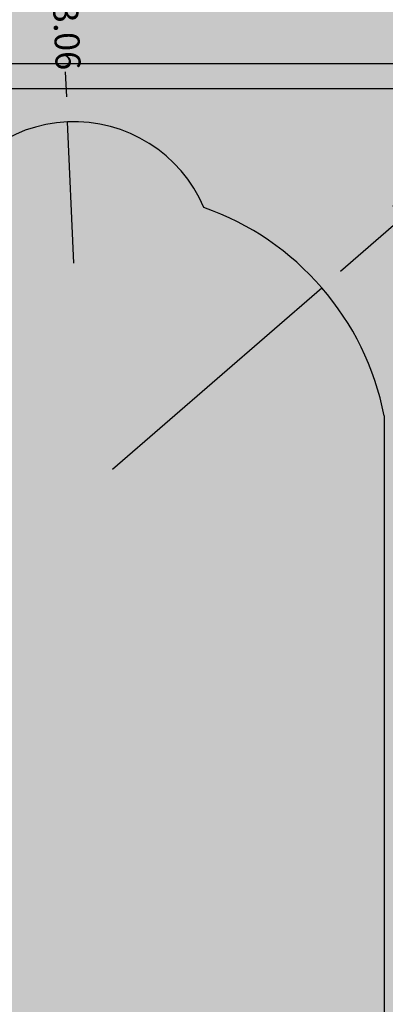
# Model space of a CAD drawing. Units: millimetres. Extents: x 78378 to 86415, y 148682 to 152721.
# Tile 8 of 18: x 80358 to 80650, y 149707 to 150495. Entities that reach past the tile are written whole.
import ezdxf

# ---------------------------------------------------------------- set-up
doc = ezdxf.new("R2010")
doc.units = ezdxf.units.MM
for name, color, linetype, lineweight in [('A-ANNO-DIMS', 2, 'Continuous', 18), ('A-FURN', 4, 'Continuous', 25), ('A-FURN-PATT', 32, 'Continuous', 13)]:
    doc.layers.add(name, color=color, linetype=linetype, lineweight=lineweight)
doc.styles.get("Standard").update_dxf_attribs({"font": 'arial.ttf'})
doc.dimstyles.new('ISO-25', dxfattribs={"dimtxt": 20, "dimasz": 20, "dimexe": 1.25, "dimexo": 0.625, "dimtad": 0, "dimdec": 1, "dimtxsty": 'Standard', "dimcen": 2.5, "dimadec": 0, "dimazin": 0, "dimtfac": 1, "dimtdec": 1, "dimtmove": 0, "dimatfit": 3, "dimfxl": 1, "dimarcsym": 0})

# ---------------------------------------------------------------- blocks, each defined once
blk = doc.blocks.new('*D32')
at = {"layer": 'A-ANNO-DIMS', "color": 0, "lineweight": -2, "transparency": 16777216}
for p, q in [((80086.404202, 150459.382643), (80086.404202, 148693.757643)), ((80692.621985, 150459.382643), (80692.621985, 148693.757643)), ((80106.404202, 148695.007643), (80355.19095843862, 148695.007643)), ((80672.621985, 148695.007643), (80423.8352285614, 148695.007643))]:
    blk.add_line(p, q, dxfattribs=at)
at = {"layer": 'A-ANNO-DIMS', "color": 0, "transparency": 16777216}
for points in [[(80106.404202, 148698.3409763333), (80106.404202, 148691.6743096666), (80086.404202, 148695.007643)], [(80672.621985, 148698.3409763333), (80672.621985, 148691.6743096666), (80692.621985, 148695.007643)]]:
    blk.add_solid(points, dxfattribs=at)
at = {"layer": 'Defpoints', "color": 0, "transparency": 16777216}
for p in [(80086.404202, 150460.007643), (80692.621985, 150460.007643), (80692.621985, 148695.007643)]:
    blk.add_point(p, dxfattribs=at)
at = {"layer": 'A-ANNO-DIMS', "color": 0, "transparency": 16777216, "insert": (80389.5130935, 148695.007643), "char_height": 20, "attachment_point": 5}
blk.add_mtext('606.2', dxfattribs=at)
blk = doc.blocks.new('*D64')
at = {"layer": 'A-ANNO-DIMS', "color": 0, "lineweight": -2, "transparency": 16777216}
for p, q in [((80660.77001983493, 150333.8066227563), (80614.48064048769, 150293.718303372)), ((80431.87671599998, 150135.576532), (80599.36214899998, 150280.625129))]:
    blk.add_line(p, q, dxfattribs=at)
at = {"layer": 'A-ANNO-DIMS', "color": 0, "transparency": 16777216}
blk.add_solid([(80612.29844475898, 150296.2380519533), (80616.66283621638, 150291.1985547907), (80599.36214899998, 150280.625129)], dxfattribs=at)
at = {"layer": 'Defpoints', "color": 0, "transparency": 16777216}
for p in [(80599.36214899998, 150280.625129), (80431.87671599998, 150135.576532)]:
    blk.add_point(p, dxfattribs=at)
at = {"layer": 'A-ANNO-DIMS', "color": 0, "transparency": 16777216, "insert": (80699.85340866249, 150367.6542870809), "char_height": 20, "attachment_point": 5, "rotation": 40.8937772563324}
blk.add_mtext('R221.56', dxfattribs=at)
blk = doc.blocks.new('*D65')
at = {"layer": 'A-ANNO-DIMS', "color": 0, "lineweight": -2, "transparency": 16777216}
for p, q in [((80394.07505015802, 150453.2874886128), (80394.982532079, 150433.3080873064)), ((80401.020132, 150300.382429), (80395.890014, 150413.328686))]:
    blk.add_line(p, q, dxfattribs=at)
at = {"layer": 'A-ANNO-DIMS', "color": 0, "transparency": 16777216}
blk.add_solid([(80398.31243229675, 150433.4593342933), (80391.65263186127, 150433.1568403196), (80395.890014, 150413.328686)], dxfattribs=at)
at = {"layer": 'Defpoints', "color": 0, "transparency": 16777216}
for p in [(80395.890014, 150413.328686), (80401.020132, 150300.382429)]:
    blk.add_point(p, dxfattribs=at)
at = {"layer": 'A-ANNO-DIMS', "color": 0, "transparency": 16777216, "insert": (80391.72908404085, 150504.937000764), "char_height": 20, "attachment_point": 5, "rotation": 272.600637092961}
blk.add_mtext('R113.06', dxfattribs=at)

msp = doc.modelspace()

# ---------------------------------------------------------------- hatches: boundary and pattern name
at = {"layer": 'A-FURN-PATT'}
h = msp.add_hatch(color=256, dxfattribs=at)
h.dxf.hatch_style = 1
h.paths.add_polyline_path([(78839.32762104142, 151040.0076434961), (78579.5199999061, 151190.0076434961), (78579.51999990609, 150470.0076434961), (78839.3276210414, 150320.0076434962)])
h.paths.add_polyline_path([(79073.15448006323, 150899.6468812434, 0.2777796948118413), (79002.26445210895, 150996.320534414, 0.7910839311940991), (78917.95668085644, 150978.871860828, 0.1804483162531181), (78856.64812911711, 150853.0137915998), (78856.6481291171, 150350.6972986685), (79073.15448006321, 150484.3179883237)])
h.paths.add_polyline_path([(79073.15448006324, 151175.0076434962), (78856.64812911711, 151050.0076434961), (78856.64812911711, 150853.0137915998, -0.1804483162531142), (78917.95668085644, 150978.871860828, -0.7910839311941295), (79002.26445210895, 150996.320534414, -0.2777796948118357), (79073.15448006323, 150899.6468812434)])
h.paths.add_polyline_path([(79341.6223552364, 151350.0076434962), (79099.13524217675, 151490.0076434961), (78596.84050798177, 151200.0076434961), (78839.32762104142, 151060.0076434961)])
h.paths.add_polyline_path([(79904.53886769625, 151675.0076434962), (79662.05175463663, 151815.0076434961), (79099.13524217677, 151490.0076434961), (79341.62235523641, 151350.0076434962)])
h.paths.add_polyline_path([(80389.51309381555, 151955.0076434962), (80389.51309381555, 152235.0076434961), (79662.05175463663, 151815.0076434961), (79904.53886769625, 151675.0076434962)])
h.paths.add_polyline_path([(80389.51309381556, 151955.0076434962), (80164.3464888316, 151825.0076434962), (80164.3464888316, 151105.0076434962), (80614.67969879952, 151105.0076434962), (80614.6796987995, 151825.0076434962)])
edge = h.paths.add_edge_path(flags=16)
edge.add_spline(control_points=[(80216.30801305865, 151728.2510436129), (80227.18536059232, 151732.9809964381), (80256.33007611947, 151745.6544105326), (80298.40995723462, 151761.9595198717), (80340.25974320961, 151805.8549546823), (80391.07708467716, 151782.0404209196), (80454.03959007034, 151805.7580622626), (80496.50068603146, 151742.4094823368), (80543.82179764508, 151733.4042954735), (80562.71817457242, 151729.808323201)], knot_values=[0, 0, 0, 0, 35.54374676083332, 95.23575346876503, 136.367675126486, 200.9329819670103, 236.7264108107793, 322.8899349763893, 380.1702736670829, 380.1702736670829, 380.1702736670829, 380.1702736670829], degree=3, periodic=0)
edge.add_line((80562.71817457242, 151729.808323201), (80562.71817457245, 151165.0076434962))
edge.add_line((80562.71817457245, 151165.0076434962), (80216.30801305866, 151165.0076434962))
edge.add_line((80216.30801305866, 151165.0076434962), (80216.30801305865, 151728.2510436129))
h.paths.add_polyline_path([(80632.00020687516, 152095.0076434962), (80389.51309381555, 152235.0076434961), (80389.51309381555, 151955.0076434962), (80614.6796987995, 151825.0076434962), (80632.0002068752, 151815.0076434962)])
h.paths.add_polyline_path([(80867.77935513339, 151958.88048878), (80632.00020687516, 152095.0076434962), (80632.0002068752, 151815.0076434962), (80632.0002068752, 151510.0076434961), (80867.77935513335, 151373.88048878)])
h.paths.add_polyline_path([(80147.02598075592, 151495.8202891389, 0.1891897896548484), (80063.56711348135, 151597.7244306894, 0.7882613551016187), (79979.26906997921, 151580.5832085911, 0.1607261321771384), (79904.53886769625, 151413.5769349066), (79904.53886769625, 150955.0076434962), (80147.0259807559, 151095.0076434962)])
h.paths.add_polyline_path([(80147.02598075592, 151815.0076434961), (79904.53886769625, 151675.0076434962), (79904.53886769625, 151413.5769349066, -0.1607261321771371), (79979.26906997921, 151580.5832085911, -0.7882613551017736), (80063.56711348135, 151597.7244306894, -0.189189789654803), (80147.02598075592, 151495.820289139)])
h.paths.add_polyline_path([(79887.21835962054, 151645.0076434962), (79640.40111954202, 151502.5076434962), (79640.40111954202, 151262.3324568555, -0.160726132177166), (79715.13132182499, 151429.33873054, -0.7882613551016538), (79799.42936532712, 151446.4799526383, -0.2129057797217132), (79887.21835962054, 151328.7246881029)])
h.paths.add_polyline_path([(79799.42936532712, 151446.4799526383, 0.7882613551016341), (79715.13132182499, 151429.33873054, 0.1607261321772164), (79640.40111954202, 151262.3324568554), (79640.401119542, 150822.5076434962), (79887.21835962054, 150965.0076434962), (79887.21835962054, 151328.7246881029, 0.2129057797217146)])
h.paths.add_polyline_path([(79605.76010339064, 151482.5076434962), (79358.94286331208, 151340.0076434962), (79358.94286331208, 151100.0700856759, -0.1607261321769527), (79433.67306559504, 151267.0763593602, -0.7882613551016573), (79517.97110909715, 151284.2175814584, -0.2129057797218584), (79605.76010339064, 151166.4623169229)])
h.paths.add_polyline_path([(79605.76010339064, 151166.4623169229, 0.2129057797218619), (79517.97110909715, 151284.2175814584, 0.7882613551016192), (79433.67306559504, 151267.0763593602, 0.160726132177026), (79358.94286331208, 151100.0700856758), (79358.9428633121, 150742.9831021798), (79419.08774136574, 150694.7323050308), (79605.76010339062, 150802.5076434962)])
edge = h.paths.add_edge_path(flags=0)
edge.add_spline(control_points=[(81152.43559504113, 151098.7675637242), (81105.72083218757, 151145.9466131586), (81038.6136018851, 151213.7208057789), (80882.38658818699, 151214.1937625951), (80797.44342369089, 151311.2996726886), (80711.86856819791, 151340.3754369685), (80681.7690729932, 151350.6023409169)], knot_values=[0, 0, 0, 0, 188.2334409997391, 270.4032751997918, 445.4517920122014, 540.4285882874335, 540.4285882874335, 540.4285882874335, 540.4285882874335], degree=3, periodic=0)
edge.add_line((80683.45384528628, 151350.0268865391), (80683.45384528628, 151104.8791667058))
edge.add_line((80683.45384528628, 151104.8791667058), (81152.43559504113, 150851.3990036113))
edge.add_line((81152.43559504113, 150851.3990036113), (81152.43559504113, 151098.7675637242))
edge = h.paths.add_edge_path(flags=0)
edge.add_spline(control_points=[(80912.90176973268, 151027.1103287246), (80892.37419951524, 151034.1027281281), (80860.16629805118, 151045.073851773), (80835.5096829066, 151068.1214310134), (80826.56785747813, 151076.4797327879)], knot_values=[0, 0, 0, 0, 63.98405104007646, 100.3914242817051, 100.3914242817051, 100.3914242817051, 100.3914242817051], degree=3, periodic=0)
edge.add_arc((80830.04136161639, 151081.2991864332), 5.940737701461331, 100.92772760250938, 234.2187380998064, ccw=False)
edge.add_spline(control_points=[(80828.91517224, 151087.1322012562), (80837.85699766847, 151078.7738994817), (80862.513612813, 151055.7263202413), (80894.72151427707, 151044.7551965964), (80915.24908449454, 151037.7627971929)], knot_values=[0, 0, 0, 0, 36.40737324162872, 100.3914242817051, 100.3914242817051, 100.3914242817051, 100.3914242817051], degree=3, periodic=0)
edge.add_arc((80914.78821288893, 151032.2794977135), 5.50263353472094, -107.95403991859422, 85.19557899478139, ccw=False)
h.paths.add_polyline_path([(81238.21798952432, 151110.0076434962), (80632.0002068752, 151460.0076434962), (80632.00020687521, 151105.0076434962), (81238.21798952432, 150755.0076434961)])
edge = h.paths.add_edge_path(flags=16)
edge.add_line((81152.43559504113, 150851.3990036113), (80683.45384528628, 151104.8791667058))
edge.add_line((80683.45384528628, 151104.8791667058), (80683.45384528628, 151350.0278851498))
edge.add_spline(control_points=[(80681.7690729932, 151350.6023409169), (80711.86856819793, 151340.3754369685), (80797.44342369087, 151311.2996726885), (80882.38658818699, 151214.1937625951), (81038.61360188508, 151213.7208057789), (81105.72083218754, 151145.9466131586), (81152.43559504113, 151098.7675637242)], knot_values=[0, 0, 0, 0, 94.97679627523202, 270.0253130876416, 352.1951472876943, 540.4285882874335, 540.4285882874335, 540.4285882874335, 540.4285882874335], degree=3, periodic=0)
edge.add_line((81152.43559504113, 151098.7675637242), (81152.43559504113, 150851.3990036113))
edge = h.paths.add_edge_path(flags=0)
edge.add_spline(control_points=[(80912.90176973268, 151027.1103287246), (80892.37419951524, 151034.1027281281), (80860.16629805118, 151045.073851773), (80835.5096829066, 151068.1214310134), (80826.56785747813, 151076.4797327879)], knot_values=[0, 0, 0, 0, 63.98405104007646, 100.3914242817051, 100.3914242817051, 100.3914242817051, 100.3914242817051], degree=3, periodic=0)
edge.add_arc((80830.04136161639, 151081.2991864332), 5.940737701461331, 100.92772760250938, 234.2187380998064, ccw=False)
edge.add_spline(control_points=[(80828.91517224, 151087.1322012562), (80837.85699766847, 151078.7738994817), (80862.513612813, 151055.7263202413), (80894.72151427707, 151044.7551965964), (80915.24908449454, 151037.7627971929)], knot_values=[0, 0, 0, 0, 36.40737324162872, 100.3914242817051, 100.3914242817051, 100.3914242817051, 100.3914242817051], degree=3, periodic=0)
edge.add_arc((80914.78821288893, 151032.2794977135), 5.50263353472094, -107.74178823087311, 85.19557899478139, ccw=False)
h.paths.add_polyline_path([(81498.02561065964, 151255.0076434964), (81238.21798952432, 151110.0076434962), (81238.21798952432, 150755.0076434961), (81498.02561065964, 150905.0076434961)])
edge = h.paths.add_edge_path(flags=16)
edge.add_spline(control_points=[(81152.43559504113, 151098.7675637242), (81105.72083218757, 151145.9466131586), (81038.6136018851, 151213.7208057789), (80882.38658818699, 151214.1937625951), (80797.44342369089, 151311.2996726886), (80711.86856819791, 151340.3754369685), (80681.7690729932, 151350.6023409169)], knot_values=[0, 0, 0, 0, 188.2334409997391, 270.4032751997918, 445.4517920122014, 540.4285882874335, 540.4285882874335, 540.4285882874335, 540.4285882874335], degree=3, periodic=0)
edge.add_line((80683.45384528628, 151350.0278851498), (80683.45384528628, 151104.8791667058))
edge.add_line((80683.45384528628, 151104.8791667058), (81152.43559504113, 150851.3990036113))
edge.add_line((81152.43559504113, 150851.3990036113), (81152.43559504113, 151098.7675637242))
h.paths.add_polyline_path([(81453.99042063669, 151280.4313723099), (80867.77935513337, 151618.8804887802), (80867.77935513335, 151373.88048878), (81238.21798952432, 151160.0076434962)])
edge = h.paths.add_edge_path(flags=16)
edge.add_line((81189.23035884998, 151297.6373231461), (81114.41656350951, 151300.215424286))
edge.add_arc((81412.09668133054, 151394.0166835757), 312.1091616570752, 179.756930250193, 197.4900342341806, ccw=False)
edge.add_ellipse((81154.0183349007, 151392.0436487034), major_axis=(-54.02641628705902, 3.630104487441717), ratio=0.22179693447735, start_angle=0, end_angle=0.351798526980474, ccw=False)
edge.add_ellipse((81154.0183349007, 151392.0436487034), major_axis=(-54.02641628705902, 3.630104487441717), ratio=0.22179693447735, start_angle=180, end_angle=359.9999999999994, ccw=False)
edge.add_spline(control_points=[(81196.1844279047, 151321.9475927373), (81224.98016894507, 151347.1455424091), (81266.88460841302, 151383.8143662904), (81222.03544587504, 151387.0303756764), (81208.00556851825, 151388.036419373)], knot_values=[0, 0, 0, 0, 75.09175173428014, 109.275804386584, 109.275804386584, 109.275804386584, 109.275804386584], degree=3, periodic=0)
edge.add_arc((80751.91118424264, 151435.614496195), 458.5692540520198, 342.489160211778, 345.646172005802, ccw=False)
edge = h.paths.add_edge_path(flags=0)
edge.add_spline(control_points=[(81196.61933933741, 151323.6570128237), (81197.89298947518, 151324.7716730423), (81199.16543060394, 151325.8857721112), (81209.0232630699, 151334.5342782859), (81217.3958880952, 151341.9835067706), (81228.09276343176, 151352.5011683344), (81231.38832729329, 151355.9523700551), (81236.9492742566, 151362.4394637984), (81239.21399888789, 151365.4773121109), (81241.49874594079, 151369.4160429918), (81242.06403714154, 151370.554153099), (81242.91869346309, 151372.6971027681), (81243.20761616631, 151373.7015371057), (81243.50116908352, 151375.5538574188), (81243.50645821408, 151376.4000030934), (81243.24316774576, 151377.9407252098), (81242.97751237078, 151378.6372898393), (81242.14015699248, 151379.9370354702), (81241.5658612394, 151380.5415506406), (81240.20389796112, 151381.5329566703), (81239.49629055885, 151381.9384109359), (81237.06189936084, 151383.0663204191), (81235.02423457924, 151383.6998500153), (81230.35196602745, 151384.7569136921), (81227.71727859117, 151385.1826462377), (81221.91180586112, 151385.9145017437), (81218.71933734383, 151386.213257908), (81213.79120700595, 151386.611489939), (81212.12519739784, 151386.7359484812), (81209.61962229511, 151386.9181059123), (81208.78653612663, 151386.9778506286), (81207.90086381555, 151387.0431786834)], knot_values=[0.0154874367935492, 0.0154874367935492, 0.0154874367935492, 0.0154874367935492, 3.337879569258078, 3.337879569258078, 25.85130624162371, 25.85130624162371, 37.52811307983364, 37.52811307983364, 49.20491991804358, 49.20491991804358, 54.285093800687, 54.285093800687, 59.36526768333043, 59.36526768333043, 64.44544156597385, 64.44544156597385, 69.52561544861727, 69.52561544861727, 74.6057893312607, 74.6057893312607, 78.49366784748545, 78.49366784748545, 86.25567095319849, 86.25567095319849, 94.01767405891154, 94.01767405891154, 102.2022655586974, 102.2022655586974, 106.2945613085904, 106.2945613085904, 108.3252217467433, 108.3252217467433, 108.3252217467433, 108.3252217467433], degree=3, periodic=0)
edge = h.paths.add_edge_path(flags=16)
edge.add_arc((81034.17317896045, 151350.4692849881), 42.58223422336468, 231.2679035139937, 306.15184603107093, ccw=False)
edge.add_line((81007.5303374241, 151317.2517344113), (81007.5303374241, 151395.1810388082))
edge.add_ellipse((81033.41196842556, 151394.7791071004), major_axis=(-25.88163100145178, 0.4537615328445103), ratio=0.2389450898152861, start_angle=0, end_angle=0.1147075293308717, ccw=False)
edge.add_ellipse((81033.41196842556, 151394.7791071004), major_axis=(-25.88163100145178, 0.4537615328445103), ratio=0.2389450898152861, start_angle=181.1677708707583, end_angle=358.9476457193874, ccw=False)
edge.add_ellipse((81033.41196842556, 151395.7791071004), major_axis=(-25.88163100145178, 0.4537615328445103), ratio=0.2389450898152861, start_angle=179.9999999981626, end_angle=360.1147075293309, ccw=False)
edge.add_ellipse((81033.41196842556, 151395.7791071004), major_axis=(-25.88163100145178, 0.4537615328445103), ratio=0.2389450898152861, start_angle=178.9476457196991, end_angle=179.9999999981626, ccw=False)
edge.add_line((81059.293599427, 151395.1778229301), (81059.293599427, 151394.3771753934))
edge.add_ellipse((81033.41196842556, 151394.7791071004), major_axis=(-25.88163100145178, 0.4537615328445103), ratio=0.2389450898152861, start_angle=179.9999999981626, end_angle=180.1147075311684, ccw=False)
edge.add_ellipse((81033.41196842556, 151394.7791071004), major_axis=(-25.88163100145178, 0.4537615328445103), ratio=0.2389450898152861, start_angle=3.6903097823663984, end_angle=176.440650305715, ccw=False)
edge.add_line((81059.293599427, 151393.3387785743), (81059.293599427, 151316.0859874871))
h.paths.add_polyline_path([(80951.93545857484, 151343.9567836094), (80909.6837602833, 151362.463470517), (80904.02186617583, 151443.961481619, -0.3813330760227573), (80987.21689667807, 151411.3716886216)], flags=16)
h = msp.add_hatch(color=256, dxfattribs=at)
h.dxf.hatch_style = 1
h.paths.add_polyline_path([(80389.81355980314, 150935.1811176149), (80389.51309381555, 151105.0076434962), (80164.3464888316, 151105.0076434962), (79904.53886769625, 150955.0076434962), (79433.58476952511, 150683.1021681411), (79459.41281351625, 150662.3818050495), (79243.9048024148, 150537.9581968276), (79160.4069246431, 150518.167363956), (78839.3276210414, 150320.0076434962), (78579.51999990609, 150470.0076434961), (78570.85974586825, 150475.0076434961), (78570.85974586825, 150465.0076434962), (78570.85974586825, 149885.0076434961)])
h.paths.add_polyline_path([(80086.40420249099, 150460.0076434961), (79826.59658135568, 150610.0076434961), (78570.85974586825, 149885.0076434961), (78830.66736700358, 149735.0076434961)])
h.paths.add_polyline_path([(79540.80006404899, 150161.0556565937), (79217.39666007676, 149974.3386142535), (78980.9165707482, 150110.8704574853), (79304.31997472048, 150297.5874998256)], flags=16)
h.paths.add_polyline_path([(79506.15904789761, 150161.0556565937), (79217.39666007677, 149994.3386142535), (79015.55758689957, 150110.8704574853), (79304.31997472048, 150277.5874998256)], flags=0)
edge = h.paths.add_edge_path(flags=0)
edge.add_arc((79247.8635885932, 150177.154059363), 137.979927152229, 256.0025927560106, 293.5594108656914)
edge.add_arc((79240.76712928673, 150078.260535577), 68.08549769177299, 336.0991039681863, 387.369687653981)
edge.add_ellipse((79258.3073696606, 150109.4851683714), major_axis=(-42.62344506003415, -1.659142297571932), ratio=0.1604284291443649, start_angle=0, end_angle=179.0977278657225, ccw=False)
edge.add_arc((79285.21118690472, 150074.2509041072), 77.20964330046426, 155.1233103751286, 203.6557939001038)
edge = h.paths.add_edge_path(flags=0)
edge.add_ellipse((79258.69578401413, 150110.8297486024), major_axis=(-42.62344506003415, -1.659142297571932), ratio=0.1604284291443649, start_angle=350.6039411592706, end_angle=356.2289762200799)
edge.add_line((79219.16897707367, 150111.8937051806), (79218.32684768032, 150109.4140931549))
edge.add_arc((79262.46751974897, 150032.9602064517), 88.28134413732826, 112.39312291994881, 119.99999999999571, ccw=False)
h.paths.add_polyline_path([(79287.06250338514, 150086.9702731333, -0.247702064009433), (79288.19674658246, 150077.2955427019, -0.3904765126137986), (79265.47309673205, 150072.5437639662, -0.4872615262363024), (79264.07897218876, 150082.3768585209, 0.3956043262328261)], flags=0)
h.paths.add_polyline_path([(80389.51309381556, 150935.0076434961), (79826.59658135568, 150610.0076434961), (80086.40420249099, 150460.0076434961), (80692.6219851401, 150460.0076434961), (80952.42960627541, 150610.0076434961)])
edge = h.paths.add_edge_path(flags=16)
edge.add_ellipse((80392.44658491029, 150825.6009587087), major_axis=(-133.0756756189512, 7.721978101297283), ratio=0.424499569836956, start_angle=0, end_angle=360)
edge = h.paths.add_edge_path(flags=0)
edge.add_spline(control_points=[(80269.35411604258, 150832.7436415815), (80269.29193278665, 150831.6720147667), (80269.35031475963, 150830.592249842), (80269.73411879689, 150828.3360718096), (80270.06118209881, 150827.1586823489), (80271.04613754865, 150824.6748448987), (80271.70517726007, 150823.3691586005), (80273.40612032128, 150820.6503360826), (80274.44810410585, 150819.2381263036), (80276.93657810257, 150816.3508564802), (80278.3827638828, 150814.8762414973), (80282.58575216534, 150811.0913237019), (80285.62609899955, 150808.7701423959), (80292.60313446997, 150804.2267034199), (80296.53882829295, 150802.0041234762), (80305.19495220963, 150797.7581273222), (80309.91505114386, 150795.7343743789), (80320.0111596611, 150791.9599857595), (80325.38703862559, 150790.2091628441), (80339.21624322617, 150786.3149836253), (80347.95776464436, 150784.3563224224), (80366.06785395242, 150781.2568288573), (80375.43585590576, 150780.1158444778), (80394.309330179, 150778.7158311894), (80403.81420373028, 150778.4568170495), (80422.465596717, 150778.8319300563), (80431.61154730739, 150779.4662025667), (80449.06079653747, 150781.5837654722), (80457.36359407243, 150783.0675039467), (80472.6698529301, 150786.7766095128), (80479.67258750588, 150789.0032721294), (80490.18936031369, 150793.2813222805), (80494.12675567923, 150795.1967122277), (80501.0145611878, 150799.188512515), (80503.9631522054, 150801.2651387212), (80508.20659370373, 150804.9015163823), (80509.7300059309, 150806.4609393726), (80512.19955536906, 150809.4942049083), (80513.14558327098, 150810.9657349426), (80514.42909982229, 150813.5430698013), (80514.84355071915, 150814.6688389962), (80515.39838138374, 150816.8624682529), (80515.5404646545, 150817.9315158847), (80515.58008082317, 150820.0980035506), (80515.47732053277, 150821.197772811), (80514.99049560675, 150823.5061778107), (80514.6046629432, 150824.7154201442), (80513.48543938114, 150827.2641302181), (80512.7510921682, 150828.6026612985), (80510.88722780815, 150831.3808578872), (80509.75776214547, 150832.8196480674), (80507.0873051963, 150835.7513330261), (80505.5466409065, 150837.243857375), (80501.06238832264, 150841.0944478958), (80497.8199298022, 150843.4575549534), (80490.4173793454, 150848.0619874995), (80486.25822277585, 150850.3037143823), (80477.14480578042, 150854.5642972019), (80472.19085006021, 150856.583496544), (80461.6274878137, 150860.3244857693), (80456.01820904585, 150862.0464562905), (80441.73317330678, 150865.8126742317), (80432.78853232553, 150867.6675482482), (80414.33909310326, 150870.5316780972), (80404.8348928345, 150871.5410542788), (80385.7706775062, 150872.6572210053), (80376.21128671143, 150872.7639759942), (80357.54439280283, 150872.0728395342), (80348.43747055416, 150871.27476178), (80331.16822413795, 150868.8299635098), (80323.00642023917, 150867.1826714935), (80309.47200145545, 150863.5363064667), (80303.8627990537, 150861.6592748057), (80293.8018064812, 150857.5400855607), (80289.35122989668, 150855.2968623192), (80282.77569843757, 150851.2345481044), (80280.34726566746, 150849.4578867352), (80276.26060564672, 150845.9127204516), (80274.60404284154, 150844.1457946164), (80272.31573199967, 150841.1242619346), (80271.53575166185, 150839.8453762844), (80270.34961441216, 150837.3878672019), (80269.94168426798, 150836.2101260174), (80269.5065140611, 150834.2814629481), (80269.3988329965, 150833.5142652193), (80269.35411604258, 150832.7436415815)], knot_values=[0, 0, 0, 0, 0.0975004598125087, 0.0975004598125087, 0.1950009196250173, 0.1950009196250173, 0.2925013794375259, 0.2925013794375259, 0.3900018392500346, 0.3900018392500346, 0.4875022990625432, 0.4875022990625432, 0.6388032241337034, 0.6388032241337034, 0.7901041492048636, 0.7901041492048636, 0.9414050742760238, 0.9414050742760238, 1.092705999347184, 1.092705999347184, 1.312817101002443, 1.312817101002443, 1.532928202657702, 1.532928202657702, 1.753039304312961, 1.753039304312961, 1.973150405968221, 1.973150405968221, 2.19326150762348, 2.19326150762348, 2.413372609278739, 2.413372609278739, 2.569860632934037, 2.569860632934037, 2.726348656589336, 2.726348656589336, 2.844186581547077, 2.844186581547077, 2.962024506504818, 2.962024506504818, 3.060233875946405, 3.060233875946405, 3.158443245387991, 3.158443245387991, 3.256652614829578, 3.256652614829578, 3.354861984271164, 3.354861984271164, 3.453071353712751, 3.453071353712751, 3.551280723154337, 3.551280723154337, 3.649490092595923, 3.649490092595923, 3.803927730406353, 3.803927730406353, 3.958365368216782, 3.958365368216782, 4.112803006027212, 4.112803006027212, 4.267240643837642, 4.267240643837642, 4.489203494974081, 4.489203494974081, 4.711166346110521, 4.711166346110521, 4.93312919724696, 4.93312919724696, 5.155092048383399, 5.155092048383399, 5.377054899519838, 5.377054899519838, 5.557853608626545, 5.557853608626545, 5.738652317733252, 5.738652317733252, 5.872395555677483, 5.872395555677483, 6.006138793621714, 6.006138793621714, 6.109604996023907, 6.109604996023907, 6.2130711984261, 6.2130711984261, 6.283185307179586, 6.283185307179586, 6.283185307179586, 6.283185307179586], degree=3, periodic=0)
edge = h.paths.add_edge_path(flags=0)
edge.add_ellipse((80392.446576265, 150825.6009639553), major_axis=(-101.8397670786795, 3.392257208815831), ratio=0.403492477068114, start_angle=0, end_angle=360)
edge = h.paths.add_edge_path(flags=0)
edge.add_ellipse((80391.1657165424, 150858.3745518381), major_axis=(9.088237780547283, -0.67334552975693), ratio=0.3513541290445306, start_angle=0, end_angle=360)
h.paths.add_polyline_path([(80952.42960627541, 150610.0076434961), (80692.62198514014, 150460.0076434962), (81361.23421645904, 150073.9841917607), (81649.96279182703, 150052.7286159431), (81766.49348583283, 150120.0076434961), (81766.49348583283, 150140.0076434961), (81564.90245463562, 150256.396279624), (81564.88840704803, 150096.1962601479), (81538.90760017018, 150111.1962859926), (81538.92165266915, 150271.3963026331)])
h.paths.add_polyline_path([(81539.035680894, 151571.3304684069), (80867.77935513339, 151958.88048878), (80867.77935513337, 151618.8804887802), (81498.02561065964, 151255.0076434964), (81498.02561065964, 150905.0076434961), (81238.21798952435, 150755.0076434961), (81538.94884401507, 150581.3806037023)])
h.paths.add_polyline_path([(81766.49348583283, 151440.0076434962), (81565.01644300755, 151556.3304684069), (81564.92963647815, 150566.38058618), (81766.49348583283, 150450.0076434962)])
edge = h.paths.add_edge_path()
edge.add_line((81564.92963647815, 150566.38058618), (81564.9136990684, 150384.628856009))
edge.add_ellipse((81552.13037602534, 150358.5718270642), major_axis=(52.62721254190076, 3.506026927036754), ratio=0.4958990548584225, start_angle=367.51697565131457, end_angle=420.0564685523974, ccw=False)
edge.add_ellipse((81552.13037602534, 150358.5718270642), major_axis=(52.62721254190076, 3.506026927036754), ratio=0.4958990548584225, start_angle=351.72974196033346, end_angle=367.51697565131457, ccw=False)
edge.add_ellipse((81552.13037602534, 150345.5015529042), major_axis=(52.62721254190076, 3.506026927036754), ratio=0.4958990548584225, start_angle=352.51169489415116, end_angle=366.30060915387577, ccw=False)
edge.add_line((81603.4463374456, 150342.2038825707), (81603.50642755294, 150340.4474978293))
edge.add_ellipse((81552.13037602534, 150332.1280359686), major_axis=(52.62721254190076, 3.506026927036754), ratio=0.4958990548584225, start_angle=353.6729654395227, end_angle=365.38679972494066, ccw=False)
edge.add_ellipse((81552.13037602534, 150332.1280359686), major_axis=(52.62721254190076, 3.506026927036754), ratio=0.4958990548584225, start_angle=350.9388331002564, end_angle=353.6729654395227)
edge.add_line((81603.86882368504, 150329.8549549892), (81604.0441546891, 150324.7301729966))
edge.add_ellipse((81552.13037602534, 150317.7418284518), major_axis=(52.62721254190076, 3.506026927036754), ratio=0.4958990548584225, start_angle=355.21767463173103, end_angle=363.85533637812415, ccw=False)
edge.add_ellipse((81552.13037602534, 150317.7418284518), major_axis=(52.62721254190076, 3.506026927036754), ratio=0.4958990548584225, start_angle=341.3250873036158, end_angle=355.21767463173103, ccw=False)
edge.add_ellipse((81552.13037602534, 150317.7418284518), major_axis=(52.62721254190076, 3.506026927036754), ratio=0.4958990548584225, start_angle=293.4661701367695, end_angle=341.3250873036158, ccw=False)
edge.add_line((81564.90566138821, 150292.9663898651), (81564.90245463562, 150256.396279624))
edge.add_line((81564.90245463562, 150256.396279624), (81766.49348583283, 150140.0076434961))
edge.add_line((81766.49348583283, 150140.0076434961), (81766.49348583283, 150450.0076434962))
edge.add_line((81766.49348583283, 150450.0076434962), (81564.92963647815, 150566.38058618))
h.paths.add_polyline_path([(81525.57129610774, 150321.5980043728), (81526.59848255829, 150321.3069082928), (81528.6771290606, 150320.947049251)])
h.paths.add_polyline_path([(81512.79027333307, 150326.1128631878), (81514.50580755486, 150325.38873887), (81512.53799543541, 150326.2678422534)])
h.paths.add_polyline_path([(81533.21477271736, 150320.1614841748), (81534.69519629495, 150319.9051905676), (81536.59953044976, 150319.755668921)])
h.paths.add_polyline_path([(81518.62200466282, 150323.6512984944), (81519.22704244989, 150323.3959129888), (81521.28902816366, 150322.8115634216)])
h.paths.add_polyline_path([(81501.21834684846, 150336.259909523), (81500.35429342867, 150338.133928838), (81499.78149159584, 150340.0493926212), (81499.50316348342, 150341.9955259773), (81499.50316348343, 150343.7256661642), (81499.75838934928, 150345.5905095656), (81500.27655404429, 150347.4549063508), (81501.05505607055, 150349.3094961287), (81501.09670215519, 150349.3936770376), (81501.13888119749, 150349.4778172982), (81500.99777251929, 150349.749637304), (81500.86282558287, 150350.0225204294), (81499.50316348342, 150355.0658001372), (81499.95910976747, 150359.5002298216), (81501.89819062682, 150363.9082666975), (81505.26528150582, 150368.1645982632), (81509.96466211145, 150372.148224724), (81515.86273756725, 150375.7458987972), (81522.79183627458, 150378.8553451273), (81530.55497651099, 150381.3881677888), (81538.93146626501, 150383.2723632221), (81538.94884401507, 150581.3806037023), (80632.00020687521, 151105.0076434962), (80389.51309381555, 151105.0076434962), (80389.81417426979, 150934.8338146148), (80952.42960627541, 150610.0076434961), (81538.92165266915, 150271.3963026331), (81538.92343538092, 150291.719410528), (81538.87516273293, 150291.7210326448), (81530.1914951021, 150292.8238998863), (81522.18015347481, 150294.6903872688), (81515.08664870211, 150297.2632955209), (81509.86347084012, 150299.9959433281), (81505.6084410237, 150303.1350709547), (81502.41902318504, 150306.608774857), (81500.3682727948, 150310.3374878268), (81499.50316348343, 150314.2358015248), (81499.50316348343, 150315.9659417118), (81499.82059494797, 150318.1159244827), (81500.4869945128, 150320.2634115907), (81501.49791650465, 150322.3940767571), (81500.48699451279, 150324.4232810552), (81499.82059494796, 150326.50388518), (81499.50316348343, 150328.6220090417), (81499.50316348343, 150330.3521492286), (81499.78149159584, 150332.3262168982), (81500.35429342862, 150334.2991697576)])
h = msp.add_hatch(color=256, dxfattribs=at)
h.dxf.hatch_style = 1
h.paths.add_polyline_path([(79090.47498813891, 151205.0076434961), (78839.32762104142, 151060.0076434961), (78839.3276210414, 150320.0076434962), (79090.4749881389, 150475.0076434961)])
h.paths.add_polyline_path([(79073.15448006324, 151175.0076434962), (79073.15448006323, 150899.6468812434, -0.0454436300045199), (79073.15448006323, 150878.5652698783), (79073.15448006321, 150484.3179883237), (78856.6481291171, 150350.6972986685), (78856.64812911711, 150814.5249476813, -0.0481571609008244), (78856.64812911711, 150853.0137915998), (78856.64812911711, 151050.0076434961)], flags=16)
h.paths.add_polyline_path([(79358.94286331208, 151340.0076434962), (79605.76010339064, 151482.5076434962), (79605.76010339062, 150802.5076434962), (79419.08774136574, 150694.7323050308), (79433.58476952511, 150683.1021681411), (79623.08061146631, 150792.5076434962), (79623.08061146631, 151512.5076434962), (79341.6223552364, 151350.0076434962), (79341.6223552364, 150756.8783555866), (79358.9428633121, 150742.9831021798)])
h.paths.add_polyline_path([(79341.6223552364, 151350.0076434962), (79090.47498813891, 151205.0076434961), (79090.4749881389, 150475.0076434961), (79160.4069246431, 150518.167363956), (79107.79549621459, 150505.6972986686), (79107.79549621459, 151195.0076434962), (79109.52754702215, 151196.0076434962), (79324.3018471607, 151320.0076434962), (79324.30184716069, 150770.7736089934), (79341.6223552364, 150756.8783555866)])
h.paths.add_polyline_path([(79887.21835962054, 151645.0076434962), (79887.21835962054, 151665.0076434962), (79623.08061146631, 151512.5076434962), (79623.08061146631, 150792.5076434962), (79887.21835962054, 150945.0076434962), (79887.21835962054, 150965.0076434962), (79640.401119542, 150822.5076434962), (79640.40111954202, 151502.5076434962)])
h.paths.add_polyline_path([(79904.53886769625, 151655.0076434962), (79887.21835962054, 151645.0076434962), (79887.21835962054, 150965.0076434962), (79904.53886769625, 150975.0076434962)])
h.paths.add_polyline_path([(80164.3464888316, 151825.0076434962), (80147.02598075592, 151815.0076434961), (80147.0259807559, 151095.0076434962), (80164.3464888316, 151105.0076434962)])
h.paths.add_polyline_path([(80632.0002068752, 151510.0076434961), (80632.0002068752, 151490.0076434962), (81238.21798952432, 151140.0076434962), (81471.60449664589, 151270.2618807845), (81453.99042063669, 151280.4313723099), (81238.21798952432, 151160.0076434962)])
h.paths.add_polyline_path([(80632.0002068752, 151490.0076434962), (80632.0002068752, 151470.0076434962), (81238.21798952432, 151120.0076434962), (81489.21857265507, 151260.092389259), (81471.60449664589, 151270.2618807845), (81238.21798952432, 151140.0076434962)])
h.paths.add_polyline_path([(80632.0002068752, 151460.0076434962), (80632.00020687521, 151105.0076434962), (81238.21798952432, 150755.0076434961), (81238.21798952432, 151110.0076434962)])
edge = h.paths.add_edge_path(flags=16)
edge.add_spline(control_points=[(80681.7690729932, 151350.6023409169), (80711.86856819793, 151340.3754369685), (80797.44342369087, 151311.2996726885), (80882.38658818699, 151214.1937625951), (81038.61360188508, 151213.7208057789), (81105.72083218754, 151145.9466131586), (81152.43559504113, 151098.7675637242)], knot_values=[0, 0, 0, 0, 94.97679627523202, 270.0253130876416, 352.1951472876943, 540.4285882874335, 540.4285882874335, 540.4285882874335, 540.4285882874335], degree=3, periodic=0)
edge.add_line((81152.43559504113, 151098.7675637242), (81152.43559504113, 150851.3990036113))
edge.add_line((81152.43559504113, 150851.3990036113), (80683.45384528628, 151104.8791667058))
edge.add_line((80683.45384528628, 151104.8791667058), (80683.45384528628, 151350.0270476502))
edge = h.paths.add_edge_path(flags=0)
edge.add_spline(control_points=[(80828.91517224, 151087.1322012562), (80837.85699766847, 151078.7738994817), (80862.513612813, 151055.7263202413), (80894.72151427707, 151044.7551965964), (80915.24908449454, 151037.7627971929)], knot_values=[0, 0, 0, 0, 36.40737324162872, 100.3914242817051, 100.3914242817051, 100.3914242817051, 100.3914242817051], degree=3, periodic=0)
edge.add_arc((80914.78821288893, 151032.2794977135), 5.50263353472094, -107.95403991859422, 85.19557899478139, ccw=False)
edge.add_spline(control_points=[(80912.90176973268, 151027.1103287246), (80892.37419951524, 151034.1027281281), (80860.16629805118, 151045.073851773), (80835.5096829066, 151068.1214310134), (80826.56785747813, 151076.4797327879)], knot_values=[0, 0, 0, 0, 63.98405104007646, 100.3914242817051, 100.3914242817051, 100.3914242817051, 100.3914242817051], degree=3, periodic=0)
edge.add_arc((80830.04136161639, 151081.2991864332), 5.940737701461332, 100.92772760250938, 234.2187380998064, ccw=False)
h.paths.add_polyline_path([(80632.0002068752, 151815.0076434962), (80614.6796987995, 151825.0076434962), (80614.67969879952, 151105.0076434962), (80632.00020687521, 151105.0076434962)])
h.paths.add_polyline_path([(81498.02561065964, 151255.0076434964), (81489.21857265507, 151260.092389259), (81238.21798952432, 151120.0076434962), (80632.0002068752, 151470.0076434962), (80632.0002068752, 151460.0076434962), (81238.21798952432, 151110.0076434962)])
h.paths.add_polyline_path([(78596.84050798177, 151200.0076434961), (78579.51999990609, 151190.0076434961), (78839.32762104142, 151040.0076434961), (78839.32762104142, 151060.0076434961)])
h.paths.add_polyline_path([(78596.84050798177, 151200.0076434961), (78579.5199999061, 151210.0076434961), (78579.5199999061, 151190.0076434961)])
h.paths.add_polyline_path([(78579.5199999061, 151210.0076434961), (78570.85974586825, 151205.0076434961), (78570.85974586825, 150475.0076434961), (78579.51999990609, 150470.0076434961)])
h = msp.add_hatch(color=256, dxfattribs=at)
h.dxf.hatch_style = 1
h.paths.add_polyline_path([(80692.6219851401, 150460.0076434961), (80086.40420249102, 150460.0076434961), (80086.40420249102, 150440.0076434962), (80692.6219851401, 150440.0076434962)])
h = msp.add_hatch(color=256, dxfattribs=at)
h.dxf.hatch_style = 1
h.paths.add_polyline_path([(80692.6219851401, 150440.0076434962), (80086.40420249102, 150440.0076434962), (80086.40420249104, 149630.0076434962), (80692.62198514013, 149614.0076434961)])
h.paths.add_polyline_path([(80293.42096661613, 150335.1041026971, -0.693913746763918), (80505.02836664302, 150344.7159628166, -0.266337996674739), (80649.3207149509, 150178.1038520679), (80649.32071495091, 149665.150500639), (80129.70547268025, 149678.8647863533), (80129.70547268025, 150178.1038520678, -0.257326206066023)], flags=16)
h.paths.add_polyline_path([(80060.4234403775, 150384.3023755343), (79809.27607328002, 150239.3023755343), (79809.27607328001, 150141.6366131478), (80060.4234403775, 150286.6366131478)])
h.paths.add_polyline_path([(80086.40420249102, 150399.3023755343), (80086.40420249102, 150440.0076434961), (79783.29531116647, 150265.0076434962), (79783.29531116647, 150224.3023755343)])
edge = h.paths.add_edge_path(flags=16)
edge.add_arc((79946.63023943067, 150348.8762810125), 10.76362312575662, -18.381796908867102, 28.033199430885304, ccw=False)
edge.add_spline(control_points=[(79956.8446621052, 150345.4819987291), (79949.48615957417, 150336.2391268092), (79933.85278209679, 150316.6023454005), (79908.95072794275, 150312.561963116), (79895.76986639632, 150310.4233556278)], knot_values=[0, 0, 0, 0, 34.22568399180864, 72.71357657474474, 72.71357657474474, 72.71357657474474, 72.71357657474474], degree=3, periodic=0)
edge.add_arc((79899.38686741845, 150314.0155032977), 5.097668219542309, 123.6496152582665, 224.8024750763005, ccw=False)
edge.add_spline(control_points=[(79896.56218517898, 150318.2590149947), (79909.86104355381, 150320.2802713686), (79934.78207045459, 150324.0679487052), (79949.34122059586, 150344.4361083294), (79956.13102493295, 150353.9350019607)], knot_values=[0, 0, 0, 0, 38.48789258293611, 72.12331911350849, 72.12331911350849, 72.12331911350849, 72.12331911350849], degree=3, periodic=0)
h.paths.add_polyline_path([(80086.40420249102, 150399.3023755343), (80060.4234403775, 150384.3023755343), (80060.4234403775, 150286.6366131478), (80086.40420249102, 150301.6366131477)], flags=17)
h.paths.add_polyline_path([(79809.27607328002, 150239.3023755343), (79783.29531116647, 150224.3023755343), (79783.29531116647, 150126.6366131478), (79809.27607328001, 150141.6366131478)])
h = msp.add_hatch(color=256, dxfattribs=at)
h.dxf.hatch_style = 1
h.paths.add_polyline_path([(80060.4234403775, 150256.6366131478), (79809.27607328001, 150111.6366131478), (79809.27607328001, 149835.822128322), (80060.4234403775, 149980.822128322)])
edge = h.paths.add_edge_path(flags=16)
edge.add_arc((79897.98743573268, 150103.5556037615), 5.172557027142873, 122.07946634250479, 231.0916038546426, ccw=False)
edge.add_spline(control_points=[(79895.24031679684, 150107.9383750026), (79905.04761058795, 150110.9384185765), (79924.63570594566, 150116.9304017735), (79948.79606586948, 150128.9973088797), (79958.12577131113, 150141.8088285447), (79961.35136162004, 150146.2381981462)], knot_values=[0, 0, 0, 0, 30.92804236988506, 61.77253950703249, 78.07166049105084, 78.07166049105084, 78.07166049105084, 78.07166049105084], degree=3, periodic=0)
edge.add_arc((79956.21022997708, 150141.1519282582), 7.231969022599169, -40.6762437318896, 44.692657332507395, ccw=False)
edge.add_spline(control_points=[(79961.6949888938, 150136.4382465157), (79958.1075446695, 150132.5465068195), (79947.5298500257, 150121.0715871927), (79924.32887046793, 150108.3481182822), (79904.61096018193, 150102.4724034792), (79894.73867114159, 150099.5305727268)], knot_values=[0, 0, 0, 0, 15.82960644688596, 46.67410358404827, 77.60214595393333, 77.60214595393333, 77.60214595393333, 77.60214595393333], degree=3, periodic=0)
h.paths.add_polyline_path([(80060.4234403775, 149950.8221283219), (79809.27607328001, 149805.822128322), (79809.27607328001, 149500.0076434962), (80060.42344037753, 149645.0076434962)])
h.paths.add_polyline_path([(80649.3207149509, 150178.1038520679, 0.2663379966747387), (80505.02836664302, 150344.7159628166, 0.6939137467639167), (80293.42096661613, 150335.1041026971, 0.2573262060660234), (80129.70547268025, 150178.1038520678), (80129.70547268025, 149678.8647863533), (80649.32071495091, 149665.150500639)])

# ---------------------------------------------------------------- linework, layer by layer
at = {"layer": 'A-FURN'}
for p, q in [((80086.40420249102, 150460.0076434961), (80692.6219851401, 150460.0076434961)), ((80086.40420249102, 150440.0076434962), (80692.6219851401, 150440.0076434962)), ((80649.3207149509, 150178.1038520678), (80649.32071495091, 149665.1505006389))]:
    msp.add_line(p, q, dxfattribs=at)
for centre, radius, start, end in [((80401.0201321819, 150300.382429083), 113.0627040584925, 23.08613834522145, 162.1153879537537), ((80431.87671631214, 150135.5765319167), 221.5636827263252, 11.06612401935919, 70.72146223627777)]:
    msp.add_arc(centre, radius, start, end, dxfattribs=at)

# ---------------------------------------------------------------- dimensions: what is measured, and where the dimension line sits
at = {"layer": 'A-ANNO-DIMS'}
dim = msp.add_radius_dim(center=(80401.020132, 150300.382429), mpoint=(80395.890014, 150413.328686), dimstyle='ISO-25', override={"dimdec": 2, "dimlfac": 1, "dimrnd": 0, "dimzin": 0, "dimdsep": 46, "dimlunit": 2}, dxfattribs=at)
dim.commit()
dim.dimension.update_dxf_attribs({"geometry": '*D65', "text_midpoint": (80391.72908404085, 150504.937000764)})
dim = msp.add_linear_dim(base=(80692.621985, 148695.007643), p1=(80086.404202, 150460.007643), p2=(80692.621985, 150460.007643), dimstyle='ISO-25', override={"dimdec": 1, "dimlfac": 1, "dimrnd": 0, "dimzin": 0, "dimdsep": 46, "dimlunit": 2}, dxfattribs=at)
dim.commit()
dim.dimension.update_dxf_attribs({"geometry": '*D32', "text_midpoint": (80389.5130935, 148695.007643)})
dim = msp.add_radius_dim(center=(80431.87671599998, 150135.576532), mpoint=(80599.36214899998, 150280.625129), dimstyle='ISO-25', override={"dimdec": 2, "dimlfac": 1, "dimrnd": 0, "dimzin": 0, "dimdsep": 46, "dimlunit": 2}, dxfattribs=at)
dim.commit()
dim.dimension.update_dxf_attribs({"geometry": '*D64', "text_midpoint": (80699.85340866249, 150367.6542870809), "dimtype": 164})

doc.saveas('drawing.dxf')
